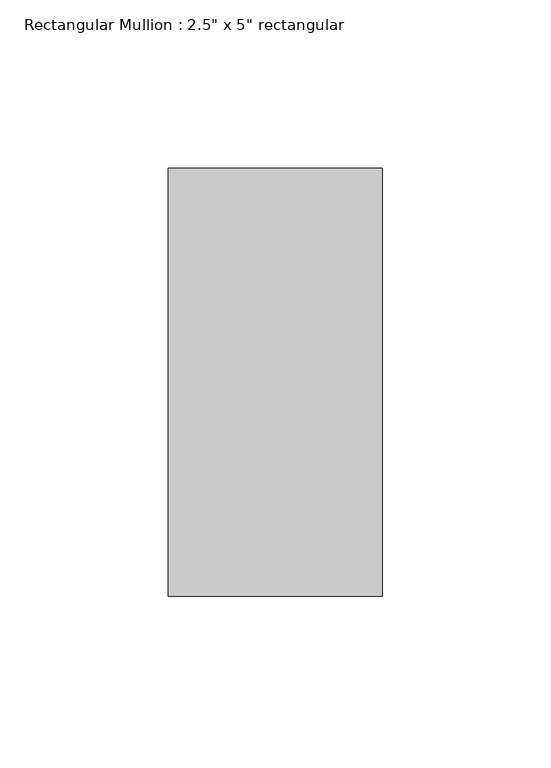
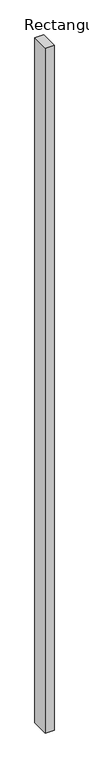
"""IFC4 building model written with IfcOpenShell, lengths in millimetres: member geometry."""

from ifc_helpers import new_model, si_unit, frame, origin, place, context, project, spatial, polyline, outline, extrude, source, transform, mapped, element, save


def member_70a47126(model_context):
    return source(origin(), model_context, "Body", "SweptSolid", [
        extrude(outline(polyline([(0.0, 63.5), (0.0, -63.5), (-63.5, -63.5), (-63.5, 63.5), (0.0, 63.5)])), frame((0.0, 0.0, -5181.6), z_axis=(0.0, 0.0, 1.0), x_axis=(1.0, 0.0, 0.0)), (0.0, 0.0, 1.0), 5181.6),
    ])


if __name__ == "__main__":
    model = new_model("IFC4")
    model_context = context("Model", 3, world=origin())
    ifc_project = project(units=[si_unit("LENGTHUNIT", "METRE", prefix="MILLI")], contexts=[model_context])
    site = spatial("IfcSite", under=ifc_project)
    building = spatial("IfcBuilding", under=site)
    placement = place(None, origin())
    member_shape = member_70a47126(model_context)
    element("IfcMember", 1, ObjectType="Rectangular Mullion : 2.5\" x 5\" rectangular", at=placement, inside=building, context=model_context, shape_type="MappedRepresentation", body=[
        mapped(member_shape, transform((0.0, 0.0, 0.0), x_axis=(1.0, 0.0, 0.0), y_axis=(0.0, 1.0, 0.0), z_axis=(0.0, 0.0, 1.0))),
    ])
    save(model, "model.ifc")

# Revit data of these elements
# Type "Rectangular Mullion : 2.5\" x 5\" rectangular"
#   built-in parameter 1007304 = 0.416667 (stored number, unit not read)
#   built-in parameter 1007301 = 0.104167 (stored number, unit not read)
#   built-in parameter 1007300 = 0.104167 (stored number, unit not read)
# Element 1 (IfcMember, "Rectangular Mullion : 2.5\" x 5\" rectangular")
#   Materials on its faces: "Iron, Ductile"
# Materials
#   "Iron, Ductile": class "Metal", colour RGB 0 0 0, transparency 0, Description = "Ductile cast iron", Cost = 0
